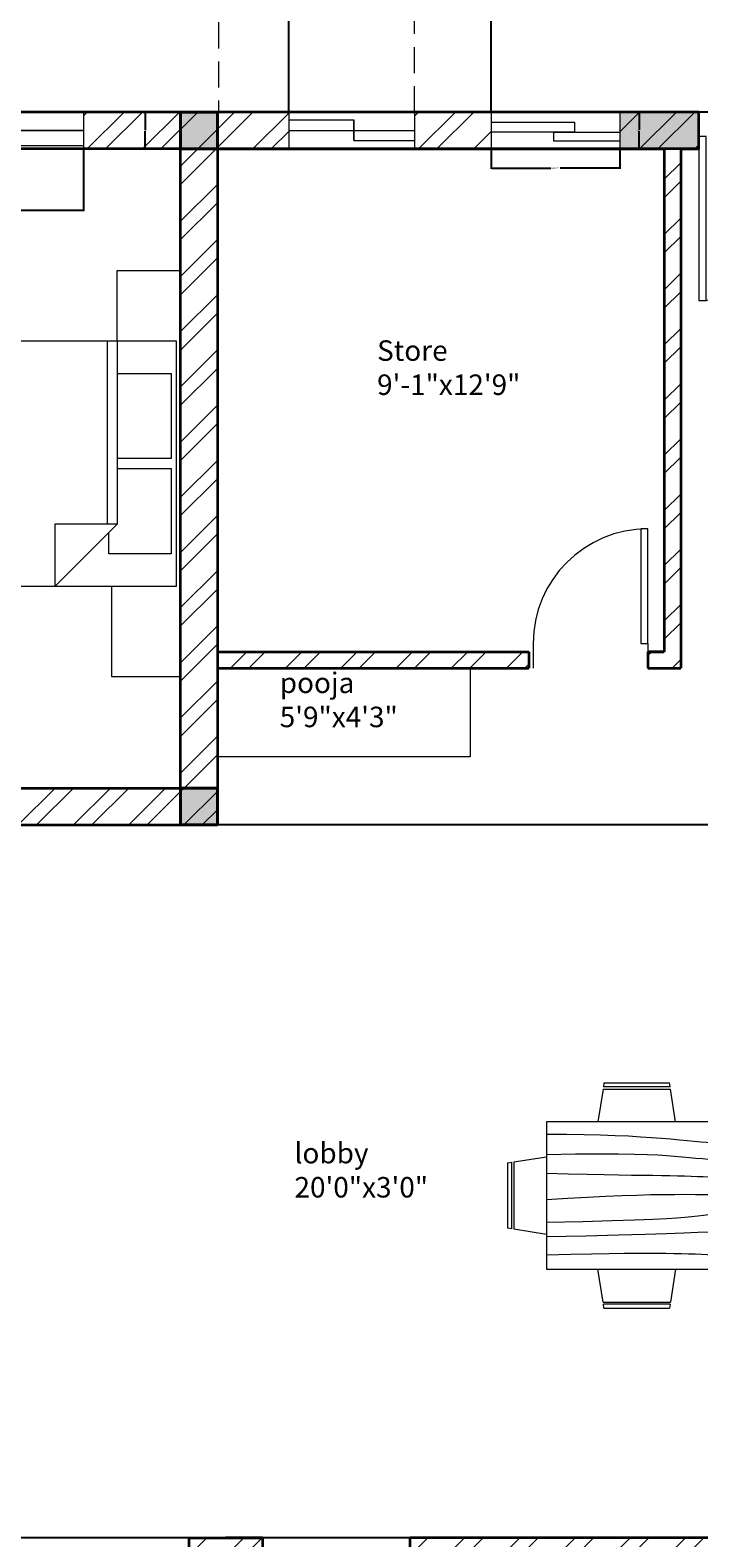
# Model space of a CAD drawing. Units: inches. Extents: x 19613 to 21413, y 12082 to 13202.
# Tile 4 of 9: x 19937 to 20100, y 12634 to 13002. Entities that reach past the tile are written whole.
import ezdxf

# ---------------------------------------------------------------- set-up
doc = ezdxf.new("R2010")
doc.units = ezdxf.units.IN
doc.linetypes.add('HIDDEN', pattern=[9.525, 6.35, -3.175])
for name, color, linetype, lineweight in [('A-ANNO-DIMS', 2, 'Continuous', 18), ('A-AREA-IDEN', 7, 'Continuous', 18), ('A-COLS', 7, 'Continuous', 40), ('A-COLS-PATT', 6, 'Continuous', 13), ('A-DOOR', 3, 'Continuous', 18), ('A-FLOR-CASE', 9, 'Continuous', 18), ('A-FLOR-HIDN', 8, 'HIDDEN', 13), ('A-FURN', 8, 'Continuous', 18), ('A-GLAZ', 4, 'Continuous', 18), ('A-WALL', 7, 'Continuous', 35), ('A-WALL-PATT', 252, 'Continuous', 13)]:
    doc.layers.add(name, color=color, linetype=linetype, lineweight=lineweight)
doc.styles.get("Standard").update_dxf_attribs({"font": 'arial.ttf'})
doc.dimstyles.get("Standard").update_dxf_attribs({"dimtxt": 0.18, "dimasz": 0.18, "dimexe": 0.18, "dimexo": 0.0625, "dimgap": 0.09, "dimtad": 0, "dimtih": 1, "dimtoh": 1, "dimdec": 4, "dimzin": 0, "dimdsep": 46, "dimtxsty": 'Standard', "dimcen": 0.09, "dimadec": 0, "dimazin": 0, "dimtfac": 1, "dimtdec": 4, "dimtofl": 0, "dimtmove": 0, "dimatfit": 3, "dimfxl": 1, "dimtolj": 1, "dimtzin": 0, "dimarcsym": 0})

# ---------------------------------------------------------------- blocks, each defined once
blk = doc.blocks.new('*U3')
for p, q in [((-28, 0), (-28, -6)), ((0, 0), (0, -6))]:
    blk.add_line(p, q)
blk.add_lwpolyline([(0, 0), (0, 28), (-1.75, 28), (-1.75, 0)], close=True)
blk.add_arc((0, 0), 28, 90, 180)
blk = doc.blocks.new('*U2')
for p, q in [((0, 0), (0, 6)), ((40, 0), (40, 6))]:
    blk.add_line(p, q)
blk.add_lwpolyline([(0, 0), (0, -40), (1.75, -40), (1.75, 0)], close=True)
blk.add_arc((0, 0), 40, 270, 0)
blk = doc.blocks.new('Bed - Queen')
for p, q in [((0, -80.00003), (0, 0)), ((0, 0), (59.99999, 0)), ((59.99999, 0), (59.99999, -80.00003)), ((7.99999, -1.2), (28.79998, -1.2)), ((7.99999, -14.4), (7.99999, -1.2)), ((28.79998, -1.2), (28.79998, -14.4)), ((31.19999, -1.2), (51.99999, -1.2)), ((31.19999, -14.4), (31.19999, -1.2)), ((51.99999, -1.2), (51.99999, -16.4)), ((0, -14.4), (44.8, -14.4)), ((59.99999, -29.6), (44.8, -14.4)), ((44.8, -14.4), (44.8, -29.6)), ((44.8, -16.8), (0, -16.8)), ((51.99999, -16.4), (46.79936, -16.4)), ((44.8, -29.6), (59.99999, -29.6)), ((59.99999, -80.00003), (0, -80.00003))]:
    blk.add_line(p, q)
blk = doc.blocks.new('Dining Set - 36 x 72 in.')
for p, q in [((-22.2343, 26.00059), (-23.4847, 17.99762)), ((-22.2304, 26), (-5.7608, 26)), ((-22, 27.5), (-22.1562, 26.50042)), ((-5.8416, 26.5), (-22.1534, 26.5)), ((-22, 27.5), (-6, 27.5)), ((-5.8437, 26.49966), (-6, 27.5)), ((-4.5152, 17.99762), (-5.7655, 25.99926)), ((5.7657, 26.00059), (4.5153, 17.99762)), ((5.7696, 26), (22.2392, 26)), ((6, 27.5), (5.8438, 26.50042)), ((22.1584, 26.5), (5.8466, 26.5)), ((6, 27.5), (22, 27.5)), ((22.1563, 26.49966), (22, 27.5)), ((23.4848, 17.99762), (22.2345, 25.99926)), ((36, 18), (-36, 18)), ((-36, 18), (-36, -18)), ((36, -18), (36, 18)), ((-45.5, 8), (-44.5004, 8.15617)), ((-45.5, 8), (-45.5, -8)), ((-44.5, -8.15843), (-44.5, 8.15338)), ((-44.0006, 8.23428), (-35.9976, 9.48474)), ((-44, 8.23041), (-44, -8.23915)), ((44.0006, 8.23428), (35.9976, 9.48474)), ((44, 8.23041), (44, -8.23915)), ((44.5, -8.15843), (44.5, 8.15338)), ((45.5, 8), (44.5005, 8.15617)), ((45.5, 8), (45.5, -8)), ((-44.4997, -8.15631), (-45.5, -8)), ((-35.9976, -9.48476), (-43.9993, -8.2345)), ((35.9976, -9.48476), (43.9993, -8.2345)), ((44.4997, -8.15631), (45.5, -8)), ((-36, -18), (36, -18)), ((-22.2343, -26.0006), (-23.4847, -17.99762)), ((-4.5152, -17.99762), (-5.7655, -25.99928)), ((5.7657, -26.0006), (4.5153, -17.99762)), ((23.4848, -17.99762), (22.2345, -25.99928)), ((-22.2304, -26), (-5.7608, -26)), ((-22, -27.5), (-22.1562, -26.50044)), ((-5.8416, -26.5), (-22.1534, -26.5)), ((-22, -27.5), (-6, -27.5)), ((-5.8437, -26.49967), (-6, -27.5)), ((5.7696, -26), (22.2392, -26)), ((6, -27.5), (5.8438, -26.50044)), ((22.1584, -26.5), (5.8466, -26.5)), ((6, -27.5), (22, -27.5)), ((22.1563, -26.49967), (22, -27.5))]:
    blk.add_line(p, q)
for points in [[(-36, 15), (-31.1772, 14.97754), (-26.8079, 14.91406), (-22.8538, 14.81543), (-19.276, 14.6875), (-16.0362, 14.53613), (-13.0957, 14.36718), (-10.4159, 14.18652), (-7.9583, 14), (-5.6904, 13.81315), (-3.6035, 13.63021), (-1.6954, 13.45508), (0.0365, 13.29166), (1.5945, 13.14388), (2.9811, 13.01562), (4.1988, 12.9108), (5.25, 12.83333), (6.1393, 12.78613), (6.8802, 12.76823), (7.4883, 12.77767), (7.9792, 12.8125), (8.3685, 12.87077), (8.6719, 12.95052), (8.9049, 13.0498), (9.0833, 13.16666), (9.2205, 13.29899), (9.3216, 13.44401), (9.3895, 13.59879), (9.4271, 13.76041), (9.4373, 13.92594), (9.4232, 14.09245), (9.3875, 14.257), (9.3333, 14.41666), (9.2638, 14.56917), (9.1836, 14.71484), (9.0975, 14.85465), (9.0104, 14.98958), (8.9272, 15.1206), (8.8529, 15.2487), (8.7922, 15.37483), (8.75, 15.5), (8.7305, 15.62467), (8.7344, 15.74739), (8.7617, 15.86621), (8.8125, 15.97916), (8.8867, 16.08431), (8.9844, 16.17968), (9.1055, 16.26334), (9.25, 16.33333), (9.4189, 16.38802), (9.6172, 16.42708), (9.8506, 16.45052), (10.125, 16.45833), (10.4463, 16.45052), (10.8203, 16.42708), (11.2529, 16.38802), (11.75, 16.33333), (12.3184, 16.26318), (12.9694, 16.17838), (13.7151, 16.07991), (14.5677, 15.96875), (15.5395, 15.84586), (16.6426, 15.71224), (17.8893, 15.56884), (19.2917, 15.41666), (20.859, 15.25667), (22.5879, 15.08984), (24.4721, 14.91715), (26.5052, 14.73958), (28.6809, 14.5581), (30.9929, 14.3737), (33.4347, 14.18733), (36, 14)], [(-36, 10), (-28.9766, 10.14274), (-23.1725, 10.20442), (-18.4241, 10.19775), (-14.5677, 10.13541), (-11.4399, 10.03011), (-8.877, 9.89453), (-6.7154, 9.74137), (-4.7917, 9.58333), (-2.9698, 9.43082), (-1.2246, 9.28515), (0.4415, 9.14534), (2.026, 9.01041), (3.5266, 8.87939), (4.9408, 8.7513), (6.266, 8.62516), (7.5, 8.5), (8.6411, 8.37549), (9.6914, 8.2539), (10.6538, 8.13818), (11.5312, 8.03125), (12.3267, 7.93603), (13.043, 7.85547), (13.6831, 7.79248), (14.25, 7.75), (14.7471, 7.7303), (15.1797, 7.73307), (15.5537, 7.75732), (15.875, 7.80208), (16.1494, 7.86637), (16.3828, 7.94922), (16.5811, 8.04964), (16.75, 8.16666), (16.8944, 8.29915), (17.0143, 8.44531), (17.1089, 8.60319), (17.1771, 8.77083), (17.218, 8.94629), (17.2305, 9.1276), (17.2137, 9.31282), (17.1667, 9.5), (17.0895, 9.6875), (16.987, 9.875), (16.8649, 10.0625), (16.7292, 10.25), (16.5856, 10.4375), (16.4401, 10.625), (16.2985, 10.8125), (16.1667, 11), (16.05, 11.18733), (15.9518, 11.3737), (15.8752, 11.5581), (15.8229, 11.73958), (15.798, 11.91715), (15.8034, 12.08984), (15.842, 12.25667), (15.9167, 12.41666), (16.0295, 12.56836), (16.1784, 12.70833), (16.3605, 12.83268), (16.5729, 12.9375), (16.8127, 13.01888), (17.0768, 13.07291), (17.3625, 13.0957), (17.6667, 13.08333), (17.9894, 13.03312), (18.3418, 12.94726), (18.7382, 12.82918), (19.1927, 12.68229), (19.7195, 12.51001), (20.3327, 12.31575), (21.0465, 12.10294), (21.875, 11.875), (22.8357, 11.63354), (23.959, 11.37304), (25.2786, 11.08618), (26.8282, 10.76562), (28.6414, 10.40405), (30.752, 9.99414), (33.1936, 9.52856), (36, 9)], [(-36, 5.5), (-30.7157, 5.3348), (-26.069, 5.20963), (-21.9946, 5.11767), (-18.4271, 5.05208), (-15.3009, 5.00602), (-12.5508, 4.97265), (-10.1112, 4.94515), (-7.9167, 4.91666), (-5.909, 4.88167), (-4.0586, 4.83984), (-2.3429, 4.79215), (-0.7396, 4.73958), (0.7739, 4.6831), (2.22, 4.6237), (3.6213, 4.56233), (5, 4.5), (6.373, 4.43782), (7.7344, 4.3776), (9.0723, 4.32129), (10.375, 4.27083), (11.6309, 4.22819), (12.8281, 4.19531), (13.9551, 4.17415), (15, 4.16666), (15.954, 4.17448), (16.819, 4.19791), (17.6001, 4.23698), (18.3021, 4.29166), (18.9299, 4.36198), (19.4883, 4.44791), (19.9823, 4.54948), (20.4167, 4.66666), (20.7969, 4.79899), (21.1302, 4.94401), (21.4245, 5.09879), (21.6875, 5.26041), (21.9271, 5.42594), (22.1511, 5.59245), (22.3672, 5.757), (22.5834, 5.91666), (22.8065, 6.06868), (23.0404, 6.21093), (23.2879, 6.34147), (23.5521, 6.45833), (23.8358, 6.55957), (24.142, 6.64323), (24.4735, 6.70735), (24.8334, 6.75), (25.2235, 6.76969), (25.642, 6.76692), (26.0858, 6.74267), (26.5521, 6.69791), (27.0379, 6.63362), (27.5404, 6.55078), (28.0565, 6.45036), (28.5834, 6.33333), (29.1242, 6.19987), (29.7071, 6.04687), (30.3661, 5.87044), (31.1354, 5.66666), (32.0493, 5.43164), (33.142, 5.16146), (34.4475, 4.85221), (36, 4.5)], [(-36, -1), (-30.7915, -0.6591), (-26.0195, -0.38216), (-21.6519, -0.16284), (-17.6563, 0.00521), (-14.0005, 0.12833), (-10.6523, 0.21289), (-7.5796, 0.26522), (-4.75, 0.29166), (-2.134, 0.29793), (0.2878, 0.28711), (2.5317, 0.26163), (4.6146, 0.22396), (6.5529, 0.17651), (8.3633, 0.12174), (10.0623, 0.06209), (11.6667, 0), (13.1899, -0.06201), (14.6341, -0.1211), (15.9982, -0.17432), (17.2813, -0.21875), (18.4823, -0.25147), (19.6003, -0.26953), (20.6343, -0.27002), (21.5834, -0.25), (22.4481, -0.20768), (23.2357, -0.14584), (23.9549, -0.06836), (24.6146, 0.02083), (25.2235, 0.11784), (25.7904, 0.21875), (26.3241, 0.31966), (26.8334, 0.41666), (27.3265, 0.50618), (27.8099, 0.58593), (28.2894, 0.65397), (28.7709, 0.70833), (29.2601, 0.74707), (29.763, 0.76823), (30.2855, 0.76985), (30.8334, 0.75), (31.4088, 0.70784), (31.9994, 0.64713), (32.589, 0.57275), (33.1615, 0.48958), (33.7008, 0.4025), (34.1908, 0.3164), (34.6153, 0.23616), (34.9584, 0.16666), (35.2099, 0.11165), (35.3848, 0.07031), (35.504, 0.04069), (35.5886, 0.02083), (35.6594, 0.00879), (35.7377, 0.0026), (35.8442, 0.00032), (36, 0)], [(-36, -6.5), (-27.1843, -6.31267), (-20.084, -6.1263), (-14.469, -5.9419), (-10.1094, -5.76042), (-6.7752, -5.58285), (-4.2363, -5.41016), (-2.2629, -5.24333), (-0.625, -5.08334), (0.8708, -4.93099), (2.2715, -4.78646), (3.5872, -4.64974), (4.8281, -4.52084), (6.0046, -4.39974), (7.127, -4.28646), (8.2053, -4.18099), (9.25, -4.08334), (10.2705, -3.99382), (11.2734, -3.91407), (12.2647, -3.84603), (13.25, -3.79167), (14.2354, -3.75293), (15.2266, -3.73177), (16.2295, -3.73015), (17.25, -3.75), (18.2912, -3.79248), (19.3451, -3.85547), (20.4009, -3.93604), (21.4479, -4.03125), (22.4754, -4.13819), (23.4727, -4.25391), (24.4289, -4.37549), (25.3334, -4.5), (26.1785, -4.62492), (26.9694, -4.74935), (27.7145, -4.87281), (28.4219, -4.99479), (29.1, -5.11483), (29.7572, -5.23242), (30.4016, -5.34709), (31.0417, -5.45834), (31.6837, -5.56437), (32.3262, -5.65821), (32.9658, -5.73153), (33.599, -5.77604), (34.2224, -5.78345), (34.8327, -5.74545), (35.4264, -5.65373), (36, -5.5)], [(-36, -10), (-26.4022, -9.81299), (-18.4675, -9.62891), (-11.9839, -9.45069), (-6.7396, -9.28125), (-2.5226, -9.12354), (0.8789, -8.98047), (3.6769, -8.85498), (6.0833, -8.75), (8.2767, -8.66765), (10.3021, -8.60677), (12.1712, -8.56543), (13.8958, -8.54167), (15.4876, -8.53353), (16.9583, -8.53907), (18.3197, -8.55632), (19.5834, -8.58334), (20.7616, -8.61841), (21.8685, -8.66081), (22.9188, -8.71004), (23.9271, -8.76563), (24.9081, -8.82707), (25.8763, -8.89388), (26.8465, -8.96558), (27.8334, -9.04167), (28.8474, -9.12118), (29.8828, -9.20117), (30.93, -9.27824), (31.9792, -9.34896), (33.0205, -9.40991), (34.0443, -9.45768), (35.0407, -9.48885), (36, -9.5)], [(-36, -14.5), (-30.0881, -14.33513), (-25.0332, -14.21224), (-20.7312, -14.12647), (-17.0781, -14.07292), (-13.97, -14.04671), (-11.3027, -14.04297), (-8.9724, -14.05681), (-6.875, -14.08334), (-4.9224, -14.11833), (-3.0905, -14.16016), (-1.3709, -14.20785), (0.2448, -14.26042), (1.7647, -14.3169), (3.1973, -14.3763), (4.5507, -14.43767), (5.8333, -14.5), (7.0554, -14.5621), (8.235, -14.62175), (9.3922, -14.67652), (10.5469, -14.72396), (11.7192, -14.76164), (12.929, -14.78711), (14.1965, -14.79794), (15.5417, -14.79167), (16.9933, -14.76424), (18.6152, -14.70508), (20.4804, -14.60197), (22.6615, -14.44271), (25.2312, -14.21509), (28.2624, -13.9069), (31.8277, -13.50594), (36, -13)]]:
    blk.add_lwpolyline(points)
blk = doc.blocks.new('*U15')
for p, q in [((0, 0), (0, 6)), ((36, 0), (36, 6))]:
    blk.add_line(p, q)
blk.add_lwpolyline([(0, 0), (0, -36), (1.75, -36), (1.75, 0)], close=True)
blk.add_arc((0, 0), 36, 270, 0)
blk = doc.blocks.new('COL-9x9')
for p, q in [((0, 9), (9, 9)), ((0, 0), (0, 9)), ((9, 9), (9, 0)), ((9, 0), (0, 0))]:
    blk.add_line(p, q)
blk = doc.blocks.new('WINDOW-BEDROOM-SLIDER')
for p, q in [((0, 9), (0, 0)), ((0, 9), (100.32, 9)), ((0, 0), (0, 9)), ((50.28, 7.85), (0, 7.85)), ((50.28, 4.5), (50.28, 7.85)), ((50.28, 7.85), (50.28, 4.5)), ((100.32, 9), (100.32, 0)), ((100.32, 9), (100.32, 0.84)), ((0, 4.5), (50.28, 4.5)), ((50.28, 4.5), (100.32, 4.5)), ((100.32, 4.5), (50.28, 4.5)), ((50.28, 4.5), (50.28, 0.84)), ((50.28, 0.84), (100.32, 0.84)), ((100.32, 0.84), (100.32, 0)), ((100.32, 0), (0, 0))]:
    blk.add_line(p, q)
blk = doc.blocks.new('WINDOW-SHORT-SLIDER-A')
for p, q in [((0, 9), (0, 0)), ((30.64, 9), (30.64, 0)), ((0, 7.09), (15.83, 7.09)), ((0, 4.5), (15.83, 4.5)), ((15.83, 4.5), (15.83, 7.09)), ((15.83, 7.09), (15.83, 4.5)), ((15.83, 4.5), (15.83, 2.04)), ((15.83, 2.04), (15.83, 4.5)), ((15.83, 4.5), (30.64, 4.5)), ((15.83, 2.04), (30.64, 2.04))]:
    blk.add_line(p, q)
blk = doc.blocks.new('WINDOW-SHORT-SLIDER-B')
for p, q in [((0, 9), (0, 0)), ((31.36, 9), (31.36, 0)), ((0, 6.5), (20.33, 6.5)), ((20.33, 4.13), (0, 4.13)), ((15.2, 4.13), (15.2, 1.96)), ((15.2, 4.13), (31.36, 4.13)), ((20.33, 6.5), (20.33, 4.13)), ((15.2, 1.96), (31.36, 1.96))]:
    blk.add_line(p, q)
blk = doc.blocks.new('*D61')
at = {"layer": 'A-ANNO-DIMS', "color": 0, "lineweight": -2, "transparency": 16777216}
for p, q in [((19849.73, 12973.22), (19849.73, 12958.05)), ((19950.05, 12973.22), (19950.05, 12958.05)), ((19849.91, 12958.23), (19898.81, 12958.23)), ((19949.87, 12958.23), (19900.98, 12958.23))]:
    blk.add_line(p, q, dxfattribs=at)
at = {"layer": 'A-ANNO-DIMS', "color": 0, "transparency": 16777216}
for points in [[(19849.91, 12958.26), (19849.91, 12958.2), (19849.73, 12958.23)], [(19949.87, 12958.26), (19949.87, 12958.2), (19950.05, 12958.23)]]:
    blk.add_solid(points, dxfattribs=at)
at = {"layer": 'Defpoints', "color": 0, "transparency": 16777216}
for p in [(19849.73, 12973.28), (19950.05, 12973.28), (19950.05, 12958.23)]:
    blk.add_point(p, dxfattribs=at)
at = {"layer": 'A-ANNO-DIMS', "color": 0, "transparency": 16777216, "insert": (19899.89, 12958.23), "char_height": 0.18, "attachment_point": 5}
blk.add_mtext('\\A1;SLIDER 100 TYP.', dxfattribs=at)
blk = doc.blocks.new('*D62')
at = {"layer": 'A-ANNO-DIMS', "color": 0, "lineweight": -2, "transparency": 16777216}
for p, q in [((19950.12, 12982.28), (19965.28, 12982.28)), ((19965.1, 12982.1), (19965.1, 12977.96)), ((19965.1, 12973.46), (19965.1, 12977.6)), ((19950.12, 12973.28), (19965.28, 12973.28))]:
    blk.add_line(p, q, dxfattribs=at)
at = {"layer": 'A-ANNO-DIMS', "color": 0, "transparency": 16777216}
for points in [[(19965.07, 12982.1), (19965.13, 12982.1), (19965.1, 12982.28)], [(19965.07, 12973.46), (19965.13, 12973.46), (19965.1, 12973.28)]]:
    blk.add_solid(points, dxfattribs=at)
at = {"layer": 'Defpoints', "color": 0, "transparency": 16777216}
for p in [(19950.05, 12982.28), (19965.1, 12982.28), (19950.05, 12973.28)]:
    blk.add_point(p, dxfattribs=at)
at = {"layer": 'A-ANNO-DIMS', "color": 0, "transparency": 16777216, "insert": (19965.1, 12977.78), "char_height": 0.18, "attachment_point": 5}
blk.add_mtext('\\A1;9 TYP.', dxfattribs=at)
blk = doc.blocks.new('*D67')
at = {"layer": 'A-ANNO-DIMS', "color": 0, "lineweight": -2, "transparency": 16777216}
for p, q in [((20049.48, 12973.22), (20049.48, 12968.4)), ((20080.84, 12973.22), (20080.84, 12968.4)), ((20049.66, 12968.58), (20064.02, 12968.58)), ((20080.66, 12968.58), (20066.29, 12968.58))]:
    blk.add_line(p, q, dxfattribs=at)
at = {"layer": 'A-ANNO-DIMS', "color": 0, "transparency": 16777216}
for points in [[(20049.66, 12968.61), (20049.66, 12968.55), (20049.48, 12968.58)], [(20080.66, 12968.61), (20080.66, 12968.55), (20080.84, 12968.58)]]:
    blk.add_solid(points, dxfattribs=at)
at = {"layer": 'Defpoints', "color": 0, "transparency": 16777216}
for p in [(20049.48, 12973.28), (20080.84, 12973.28), (20080.84, 12968.58)]:
    blk.add_point(p, dxfattribs=at)
at = {"layer": 'A-ANNO-DIMS', "color": 0, "transparency": 16777216, "insert": (20065.16, 12968.58), "char_height": 0.18, "attachment_point": 5}
blk.add_mtext('\\A1;SLIDER B 31 TYP.', dxfattribs=at)
blk = doc.blocks.new('*D68')
at = {"layer": 'A-ANNO-DIMS', "color": 0, "lineweight": -2, "transparency": 16777216}
for p, q in [((20080.9, 12982.28), (20085.72, 12982.28)), ((20085.54, 12982.1), (20085.54, 12977.96)), ((20085.54, 12973.46), (20085.54, 12977.6)), ((20080.9, 12973.28), (20085.72, 12973.28))]:
    blk.add_line(p, q, dxfattribs=at)
at = {"layer": 'A-ANNO-DIMS', "color": 0, "transparency": 16777216}
for points in [[(20085.51, 12982.1), (20085.57, 12982.1), (20085.54, 12982.28)], [(20085.51, 12973.46), (20085.57, 12973.46), (20085.54, 12973.28)]]:
    blk.add_solid(points, dxfattribs=at)
at = {"layer": 'Defpoints', "color": 0, "transparency": 16777216}
for p in [(20080.84, 12982.28), (20085.54, 12982.28), (20080.84, 12973.28)]:
    blk.add_point(p, dxfattribs=at)
at = {"layer": 'A-ANNO-DIMS', "color": 0, "transparency": 16777216, "insert": (20085.54, 12977.78), "char_height": 0.18, "attachment_point": 5}
blk.add_mtext('\\A1;9 TYP.', dxfattribs=at)
blk = doc.blocks.new('*D89')
at = {"layer": 'A-ANNO-DIMS', "color": 0, "lineweight": -2, "transparency": 16777216}
for p, q in [((20807.37, 12808.28), (19613.26, 12808.28)), ((19613.44, 12808.1), (19613.44, 12721.46)), ((19613.44, 12634.46), (19613.44, 12721.1)), ((20807.37, 12634.28), (19613.26, 12634.28))]:
    blk.add_line(p, q, dxfattribs=at)
at = {"layer": 'A-ANNO-DIMS', "color": 0, "transparency": 16777216}
for points in [[(19613.41, 12808.1), (19613.47, 12808.1), (19613.44, 12808.28)], [(19613.41, 12634.46), (19613.47, 12634.46), (19613.44, 12634.28)]]:
    blk.add_solid(points, dxfattribs=at)
at = {"layer": 'Defpoints', "color": 0, "transparency": 16777216}
for p in [(19613.44, 12808.28), (20807.43, 12808.28), (20807.43, 12634.28)]:
    blk.add_point(p, dxfattribs=at)
at = {"layer": 'A-ANNO-DIMS', "color": 0, "transparency": 16777216, "insert": (19613.44, 12721.28), "char_height": 0.18, "attachment_point": 5}
blk.add_mtext('\\A1;174', dxfattribs=at)
blk = doc.blocks.new('*D90')
at = {"layer": 'A-ANNO-DIMS', "color": 0, "lineweight": -2, "transparency": 16777216}
for p, q in [((20807.37, 12982.28), (19613.26, 12982.28)), ((19613.44, 12982.1), (19613.44, 12895.46)), ((19613.44, 12808.46), (19613.44, 12895.1)), ((20807.37, 12808.28), (19613.26, 12808.28))]:
    blk.add_line(p, q, dxfattribs=at)
at = {"layer": 'A-ANNO-DIMS', "color": 0, "transparency": 16777216}
for points in [[(19613.41, 12982.1), (19613.47, 12982.1), (19613.44, 12982.28)], [(19613.41, 12808.46), (19613.47, 12808.46), (19613.44, 12808.28)]]:
    blk.add_solid(points, dxfattribs=at)
at = {"layer": 'Defpoints', "color": 0, "transparency": 16777216}
for p in [(19613.44, 12982.28), (20807.43, 12982.28), (20807.43, 12808.28)]:
    blk.add_point(p, dxfattribs=at)
at = {"layer": 'A-ANNO-DIMS', "color": 0, "transparency": 16777216, "insert": (19613.44, 12895.28), "char_height": 0.18, "attachment_point": 5}
blk.add_mtext('\\A1;174', dxfattribs=at)
blk = doc.blocks.new('*D102')
at = {"layer": 'A-ANNO-DIMS', "color": 0, "lineweight": -2, "transparency": 16777216}
for p, q in [((19849.73, 12982.34), (19849.73, 13201.71)), ((19849.91, 13201.53), (19924.46, 13201.53)), ((19999.93, 13201.53), (19925.37, 13201.53)), ((20000.11, 12982.34), (20000.11, 13201.71))]:
    blk.add_line(p, q, dxfattribs=at)
at = {"layer": 'A-ANNO-DIMS', "color": 0, "transparency": 16777216}
for points in [[(19849.91, 13201.56), (19849.91, 13201.5), (19849.73, 13201.53)], [(19999.93, 13201.56), (19999.93, 13201.5), (20000.11, 13201.53)]]:
    blk.add_solid(points, dxfattribs=at)
at = {"layer": 'Defpoints', "color": 0, "transparency": 16777216}
for p in [(20000.11, 13201.53), (19849.73, 12982.28), (20000.11, 12982.28)]:
    blk.add_point(p, dxfattribs=at)
at = {"layer": 'A-ANNO-DIMS', "color": 0, "transparency": 16777216, "insert": (19924.92, 13201.53), "char_height": 0.18, "attachment_point": 5}
blk.add_mtext('\\A1;150.37', dxfattribs=at)
blk = doc.blocks.new('*D103')
at = {"layer": 'A-ANNO-DIMS', "color": 0, "lineweight": -2, "transparency": 16777216}
for p, q in [((20000.11, 12982.34), (20000.11, 13201.71)), ((20000.29, 13201.53), (20024.4, 13201.53)), ((20049.3, 13201.53), (20025.19, 13201.53)), ((20049.48, 12982.34), (20049.48, 13201.71))]:
    blk.add_line(p, q, dxfattribs=at)
at = {"layer": 'A-ANNO-DIMS', "color": 0, "transparency": 16777216}
for points in [[(20000.29, 13201.56), (20000.29, 13201.5), (20000.11, 13201.53)], [(20049.3, 13201.56), (20049.3, 13201.5), (20049.48, 13201.53)]]:
    blk.add_solid(points, dxfattribs=at)
at = {"layer": 'Defpoints', "color": 0, "transparency": 16777216}
for p in [(20049.48, 13201.53), (20000.11, 12982.28), (20049.48, 12982.28)]:
    blk.add_point(p, dxfattribs=at)
at = {"layer": 'A-ANNO-DIMS', "color": 0, "transparency": 16777216, "insert": (20024.79, 13201.53), "char_height": 0.18, "attachment_point": 5}
blk.add_mtext('\\A1;49.37', dxfattribs=at)

msp = doc.modelspace()

# ---------------------------------------------------------------- hatches: boundary and pattern name
at = {"layer": 'A-COLS-PATT'}
h = msp.add_hatch(color=256, dxfattribs=at)
h.dxf.hatch_style = 1
h.paths.add_polyline_path([(19701.1937, 13118.279), (19696.6937, 13118.279), (19696.6937, 13113.779), (19701.1937, 13113.779)])
h.paths.add_polyline_path([(19714.6694, 12982.279), (19705.6937, 12982.279), (19705.6937, 12973.279), (19714.6694, 12973.279)])
h.paths.add_polyline_path([(19827.1183, 12982.279), (19818.1183, 12982.279), (19818.1183, 12973.279), (19827.1183, 12973.279)])
h.paths.add_polyline_path([(19982.6937, 12982.279), (19973.6937, 12982.279), (19973.6937, 12973.279), (19982.6937, 12973.279)])
h.paths.add_polyline_path([(19982.6937, 12817.279), (19973.6937, 12817.279), (19973.6937, 12808.279), (19982.6937, 12808.279)])
h.paths.add_polyline_path([(19795.361, 12817.279), (19786.361, 12817.279), (19786.361, 12808.279), (19795.361, 12808.279)])
h.paths.add_polyline_path([(19705.6937, 12817.279), (19702.0819, 12817.279), (19702.0819, 12808.279), (19705.6937, 12808.279)])
h.paths.add_polyline_path([(19711.0819, 12817.279), (19705.6937, 12817.279), (19705.6937, 12808.279), (19711.0819, 12808.279)])
h.paths.add_polyline_path([(19714.6136, 12634.279), (19705.6937, 12634.279), (19705.6937, 12625.279), (19714.6136, 12625.279)])
h.paths.add_polyline_path([(19705.6937, 12485.8897), (19701.1937, 12485.8897), (19701.1937, 12476.8897), (19705.6937, 12476.8897)])
h.paths.add_polyline_path([(19709.3479, 12485.8897), (19705.6937, 12485.8897), (19705.6937, 12476.8897), (19709.3479, 12476.8897)])
h.paths.add_polyline_path([(19701.1937, 12485.8897), (19700.3479, 12485.8897), (19700.3479, 12476.8897), (19701.1937, 12476.8897)])
h.paths.add_polyline_path([(20218.6937, 12421.279), (20209.6937, 12421.279), (20209.6937, 12412.279), (20218.6937, 12412.279)])
h.paths.add_polyline_path([(20218.6937, 12634.279), (20209.6937, 12634.279), (20209.6937, 12625.279), (20218.6937, 12625.279)])
h.paths.add_polyline_path([(20218.6937, 12808.279), (20209.6937, 12808.279), (20209.6937, 12803.279), (20218.6937, 12803.279)])
h.paths.add_polyline_path([(20218.6937, 12810.1878), (20209.6937, 12810.1878), (20209.6937, 12808.279), (20218.6937, 12808.279)])
h.paths.add_polyline_path([(20218.6937, 12803.279), (20209.6937, 12803.279), (20209.6937, 12801.1878), (20218.6937, 12801.1878)])
h.paths.add_polyline_path([(20218.6937, 12982.279), (20209.6937, 12982.279), (20209.6937, 12973.279), (20218.6937, 12973.279)])
h.paths.add_polyline_path([(20100.1214, 12982.279), (20080.8386, 12982.279), (20080.8386, 12973.279), (20091.6937, 12973.279), (20100.1214, 12973.279), (20100.1214, 12976.279)])
h.paths.add_polyline_path([(19851.5503, 12631.279), (19851.5503, 12634.279), (19828.8814, 12634.279), (19828.8814, 12625.279), (19851.5503, 12625.279)])
at = {"layer": 'A-WALL-PATT'}
h = msp.add_hatch(dxfattribs=at)
h.set_pattern_fill('ANSI32', color=256)
h.paths.add_polyline_path([(20223.1937, 13118.279), (20218.6937, 13118.279), (19701.1937, 13118.279), (19701.1937, 13113.779), (20223.1937, 13113.779)])
h.paths.add_polyline_path([(19849.7315, 12982.279), (19799.9854, 12982.279), (19799.9854, 12973.279), (19849.7315, 12973.279)])
h.paths.add_polyline_path([(19755.5378, 12982.279), (19705.6937, 12982.279), (19705.6937, 12973.279), (19755.5378, 12973.279)])
h.paths.add_polyline_path([(20000.1054, 12982.279), (19950.0534, 12982.279), (19950.0534, 12974.1171), (19950.0534, 12973.279), (20000.1054, 12973.279)])
h.paths.add_polyline_path([(20049.4797, 12982.279), (20030.7476, 12982.279), (20030.7476, 12973.279), (20049.4797, 12973.279)])
h.paths.add_polyline_path([(20100.1214, 12982.279), (20080.8386, 12982.279), (20080.8386, 12973.279), (20100.1214, 12973.279), (20100.1214, 12976.279)])
h.paths.add_polyline_path([(20218.6937, 12982.279), (20167.6937, 12982.279), (20140.1214, 12982.279), (20140.1214, 12976.279, -0.01769781), (20140.0212, 12973.45), (20167.6937, 12973.279), (20176.6937, 12973.279), (20218.6937, 12973.279)])
h.paths.add_polyline_path([(19851.5503, 12814.279), (19851.5503, 12817.279), (19793.6937, 12817.279), (19789.6937, 12817.279), (19705.6937, 12817.279), (19705.6937, 12808.279), (19851.5503, 12808.279)])
h.paths.add_polyline_path([(19982.6937, 12973.279), (19973.6937, 12973.279), (19973.6937, 12817.279), (19887.5503, 12817.279), (19887.5503, 12808.279), (19973.6937, 12808.279), (19982.6937, 12808.279)])
h.paths.add_polyline_path([(20058.6937, 12850.5529), (19982.6937, 12850.5529), (19982.6937, 12846.5529), (20058.6937, 12846.5529)])
h.paths.add_polyline_path([(20095.6937, 12973.279), (20091.6937, 12973.279), (20091.6937, 12850.5529), (20087.6937, 12850.5529), (20087.6937, 12846.5529), (20095.6937, 12846.5529)])
h.paths.add_polyline_path([(20218.6937, 12808.279), (20140.8605, 12808.279), (20126.9413, 12808.279), (20126.9413, 12803.279), (20140.8605, 12803.279), (20218.6937, 12803.279)])
h.paths.add_polyline_path([(19738.3931, 12634.279), (19705.6937, 12634.279), (19705.6937, 12625.279), (19738.3931, 12625.279)])
h.paths.add_polyline_path([(19912.6937, 12634.279), (19903.6937, 12634.279), (19891.5503, 12634.279), (19891.5503, 12625.279), (19903.6937, 12625.279), (19903.6937, 12445.279), (19975.6937, 12445.279), (20128.6937, 12445.279), (20128.6937, 12412.279), (20149.8479, 12412.279), (20149.8479, 12421.279), (20137.6937, 12421.279), (20137.6937, 12454.279), (20137.6937, 12580.2801), (20133.6937, 12580.2801), (20133.6937, 12454.279), (19984.6937, 12454.279), (19984.6937, 12625.279), (19993.6937, 12625.279), (19993.6937, 12634.279), (19984.6937, 12634.279), (19975.6937, 12634.279), (19975.6937, 12454.279), (19912.6937, 12454.279)])
h.paths.add_polyline_path([(20218.6937, 12634.279), (20137.6937, 12634.279), (20029.6937, 12634.279), (20029.6937, 12625.279), (20137.6937, 12625.279), (20218.6937, 12625.279)])
h.paths.add_polyline_path([(21014.4339, 12634.279), (21005.4339, 12634.279), (20993.2905, 12634.279), (20993.2905, 12625.279), (21005.4339, 12625.279), (21005.4339, 12445.279), (21077.4339, 12445.279), (21230.4339, 12445.279), (21230.4339, 12412.279), (21251.5881, 12412.279), (21251.5881, 12421.279), (21239.4339, 12421.279), (21239.4339, 12454.279), (21239.4339, 12580.2801), (21235.4339, 12580.2801), (21235.4339, 12454.279), (21086.4339, 12454.279), (21086.4339, 12625.279), (21095.4339, 12625.279), (21095.4339, 12634.279), (21086.4339, 12634.279), (21077.4339, 12634.279), (21077.4339, 12454.279), (21014.4339, 12454.279)])
h.paths.add_polyline_path([(20840.1333, 12634.279), (20807.4339, 12634.279), (20807.4339, 12625.279), (20840.1333, 12625.279)])
h.paths.add_polyline_path([(20953.2905, 12631.279), (20953.2905, 12634.279), (20930.6216, 12634.279), (20930.6216, 12625.279), (20953.2905, 12625.279)])
h.paths.add_polyline_path([(21320.4339, 12634.279), (21239.4339, 12634.279), (21131.4339, 12634.279), (21131.4339, 12625.279), (21239.4339, 12625.279), (21320.4339, 12625.279)])
h.paths.add_polyline_path([(21084.4339, 12973.279), (21075.4339, 12973.279), (21075.4339, 12817.279), (20989.2905, 12817.279), (20989.2905, 12808.279), (21075.4339, 12808.279), (21084.4339, 12808.279)])
h.paths.add_polyline_path([(21142.1261, 12863.2893), (21084.4339, 12863.2893), (21084.4339, 12846.5529), (21142.1261, 12846.5529)])
h.paths.add_polyline_path([(21320.4339, 12808.279), (21242.6007, 12808.279), (21228.6815, 12808.279), (21228.6815, 12803.279), (21242.6007, 12803.279), (21320.4339, 12803.279)])
h.paths.add_polyline_path([(20857.278, 12982.279), (20807.4339, 12982.279), (20807.4339, 12973.279), (20857.278, 12973.279)])
h.paths.add_polyline_path([(20951.4717, 12982.279), (20901.7255, 12982.279), (20901.7255, 12973.279), (20951.4717, 12973.279)])
h.paths.add_polyline_path([(21101.8455, 12982.279), (21051.7936, 12982.279), (21051.7936, 12974.1171), (21051.7936, 12973.279), (21101.8455, 12973.279)])
h.paths.add_polyline_path([(21151.2199, 12982.279), (21132.4878, 12982.279), (21132.4878, 12973.279), (21151.2199, 12973.279)])
h.paths.add_polyline_path([(21201.8616, 12982.279), (21182.5788, 12982.279), (21182.5788, 12973.279), (21193.4339, 12973.279), (21201.8616, 12973.279), (21201.8616, 12976.279)])
h.paths.add_polyline_path([(21320.4339, 12982.279), (21269.4339, 12982.279), (21241.8616, 12982.279), (21241.8616, 12976.279, -0.01769781), (21241.7614, 12973.45), (21269.4339, 12973.279), (21278.4339, 12973.279), (21320.4339, 12973.279)])
h.paths.add_polyline_path([(20953.2905, 12817.279), (20895.4339, 12817.279), (20891.4339, 12817.279), (20807.4339, 12817.279), (20807.4339, 12808.279), (20953.2905, 12808.279)])
h.paths.add_polyline_path([(21197.4339, 12973.279), (21193.4339, 12973.279), (21193.4339, 12850.5529), (21197.4339, 12850.5529)])
h.paths.add_polyline_path([(21320.4339, 12550.279), (21272.5278, 12550.279), (21272.5278, 12546.279), (21320.4339, 12546.279)])
h.paths.add_polyline_path([(21320.4339, 12421.279), (21283.2222, 12421.279), (21283.2222, 12412.279), (21320.4339, 12412.279)])

# ---------------------------------------------------------------- linework, layer by layer
at = {"layer": 'A-FLOR-CASE'}
for p, q in [((20044.3114, 12846.5529), (20044.3114, 12824.8677)), ((20044.3114, 12824.8677), (19982.6937, 12824.8677))]:
    msp.add_line(p, q, dxfattribs=at)
at = {"layer": 'A-FLOR-HIDN'}
for p, q in [((19982.958, 13042.279), (19982.958, 12982.279)), ((20030.7476, 12982.279), (20030.7476, 13021.8552))]:
    msp.add_line(p, q, dxfattribs=at)
at = {"layer": 'A-FURN'}
for p, q in [((19958.2501, 12926.479), (19958.2501, 12943.6155)), ((19958.2501, 12943.6155), (19973.6937, 12943.6155)), ((19956.8662, 12866.479), (19956.8662, 12844.5201)), ((19956.8662, 12844.5201), (19973.6937, 12844.5201))]:
    msp.add_line(p, q, dxfattribs=at)
at = {"layer": 'A-WALL'}
for p, q in [((20100.1214, 12982.279), (19799.9854, 12982.279)), ((20100.1214, 12973.279), (20100.1214, 12982.279)), ((20100.1214, 12973.279), (19799.9854, 12973.279)), ((19973.6937, 12973.279), (19982.6937, 12973.279)), ((19982.6937, 12973.279), (19982.6937, 12808.279)), ((19982.6937, 12973.279), (20091.6937, 12973.279)), ((19982.6937, 12973.279), (20091.6937, 12973.279)), ((20091.6937, 12973.279), (20091.6937, 12850.5529)), ((20095.6937, 12973.279), (20095.6937, 12846.5529)), ((20095.6937, 12973.279), (20100.1214, 12973.279)), ((20095.6937, 12973.279), (20100.1214, 12973.279)), ((19982.6937, 12850.5529), (20058.6937, 12850.5529)), ((20058.6937, 12850.5529), (20058.6937, 12846.5529)), ((20091.6937, 12850.5529), (20087.6937, 12850.5529)), ((20087.6937, 12850.5529), (20087.6937, 12846.5529)), ((20087.6937, 12850.5529), (20091.6937, 12850.5529)), ((19982.6937, 12846.5529), (20058.6937, 12846.5529)), ((20087.6937, 12846.5529), (20095.6937, 12846.5529)), ((19887.5503, 12808.279), (19973.6937, 12808.279)), ((19982.6937, 12808.279), (19973.6937, 12808.279)), ((19975.6937, 12634.279), (19975.6937, 12454.279)), ((19975.6937, 12634.279), (19984.6937, 12634.279)), ((19984.6937, 12634.279), (19993.6937, 12634.279)), ((19993.6937, 12634.279), (19984.6937, 12634.279)), ((19993.6937, 12634.279), (19993.6937, 12625.279)), ((20137.6937, 12634.279), (20029.6937, 12634.279)), ((20029.6937, 12625.279), (20029.6937, 12634.279))]:
    msp.add_line(p, q, dxfattribs=at)
msp.add_lwpolyline([(19887.5503, 12817.279), (19973.6937, 12817.279), (19973.6937, 12973.279), (19799.9854, 12973.279)], dxfattribs=at)

# ---------------------------------------------------------------- block references
at = {"layer": 'A-COLS', "rotation": 180}
for p in [(19982.6941, 12982.279), (19982.6941, 12817.279)]:
    msp.add_blockref('COL-9x9', p, dxfattribs=at)
at = {"layer": 'A-DOOR'}
for name, p in [('*U2', (20100.1214, 12976.279)), ('*U3', (20087.6937, 12852.5529)), ('*U15', (19993.6937, 12628.279))]:
    msp.add_blockref(name, p, dxfattribs=at)
at = {"layer": 'A-FURN', "rotation": 270.0000000000108}
msp.add_blockref('Bed - Queen', (19972.6501, 12926.479), dxfattribs=at)
at = {"layer": 'A-FURN'}
msp.add_blockref('Dining Set - 36 x 72 in.', (20098.9872, 12717.8276), dxfattribs=at)
at = {"layer": 'A-GLAZ'}
for name, p in [('WINDOW-BEDROOM-SLIDER', (19849.732, 12973.279)), ('WINDOW-SHORT-SLIDER-A', (20000.105, 12973.279)), ('WINDOW-SHORT-SLIDER-B', (20049.48, 12973.279))]:
    msp.add_blockref(name, p, dxfattribs=at)

# ---------------------------------------------------------------- texts
at = {"layer": 'A-AREA-IDEN', "char_height": 5, "attachment_point": 1}
for s, insert in [('Store \\P9\'-1"x12\'9"', (20021.6454, 12926.5631)), ('pooja\\P5\'9"x4\'3"', (19997.8914, 12845.4755)), ('lobby\\P20\'0"x3\'0"', (20001.4975, 12730.681))]:
    msp.add_mtext_dynamic_manual_height_columns(s, width=19.652904, gutter_width=12.5, heights=[0], dxfattribs=dict(at, insert=insert))

# ---------------------------------------------------------------- dimensions: what is measured, and where the dimension line sits
at = {"layer": 'A-ANNO-DIMS'}
for base, p1, p2, picture, middle in [((20000.1054, 13201.529), (19849.7315, 12982.279), (20000.1054, 12982.279), '*D102', (19924.9185, 13201.529)), ((20049.4797, 13201.529), (20000.1054, 12982.279), (20049.4797, 12982.279), '*D103', (20024.7925, 13201.529))]:
    dim = msp.add_linear_dim(base=base, p1=p1, p2=p2, dimstyle='Standard', override={"dimdec": 2, "dimlfac": 1, "dimrnd": 0, "dimzin": 0, "dimdsep": 46, "dimlunit": 2}, dxfattribs=at)
    dim.commit()
    dim.dimension.update_dxf_attribs({"geometry": picture, "text_midpoint": middle})
for base, p1, p2, picture, middle in [((19613.4437, 12982.279), (20807.4339, 12808.279), (20807.4328, 12982.279), '*D90', (19613.4437, 12895.279)), ((19613.4437, 12808.279), (20807.4339, 12634.279), (20807.4339, 12808.279), '*D89', (19613.4437, 12721.279))]:
    dim = msp.add_linear_dim(base=base, p1=p1, p2=p2, angle=90, dimstyle='Standard', override={"dimdec": 0, "dimlfac": 1, "dimrnd": 0, "dimzin": 0, "dimdsep": 46, "dimlunit": 2}, dxfattribs=at)
    dim.commit()
    dim.dimension.update_dxf_attribs({"geometry": picture, "text_midpoint": middle})
for base, p1, p2, picture, middle in [((19965.1016, 12982.279), (19950.0534, 12973.279), (19950.0534, 12982.279), '*D62', (19965.1016, 12977.779)), ((20085.5425, 12982.279), (20080.8386, 12973.279), (20080.8386, 12982.279), '*D68', (20085.5425, 12977.779))]:
    dim = msp.add_linear_dim(base=base, p1=p1, p2=p2, angle=90, text='<> TYP.', dimstyle='Standard', override={"dimdec": 0, "dimlfac": 1, "dimrnd": 0, "dimzin": 0, "dimdsep": 46, "dimlunit": 2}, dxfattribs=at)
    dim.commit()
    dim.dimension.update_dxf_attribs({"geometry": picture, "text_midpoint": middle})
for base, p1, p2, text, picture, middle in [((19950.0534, 12958.2307), (19849.7315, 12973.279), (19950.0534, 12973.279), 'SLIDER <> TYP.', '*D61', (19899.8925, 12958.2307)), ((20080.8386, 12968.5752), (20049.4797, 12973.279), (20080.8386, 12973.279), 'SLIDER B <> TYP.', '*D67', (20065.1592, 12968.5752))]:
    dim = msp.add_linear_dim(base=base, p1=p1, p2=p2, text=text, dimstyle='Standard', override={"dimdec": 0, "dimlfac": 1, "dimrnd": 0, "dimzin": 0, "dimdsep": 46, "dimlunit": 2}, dxfattribs=at)
    dim.commit()
    dim.dimension.update_dxf_attribs({"geometry": picture, "text_midpoint": middle})

doc.saveas('drawing.dxf')
